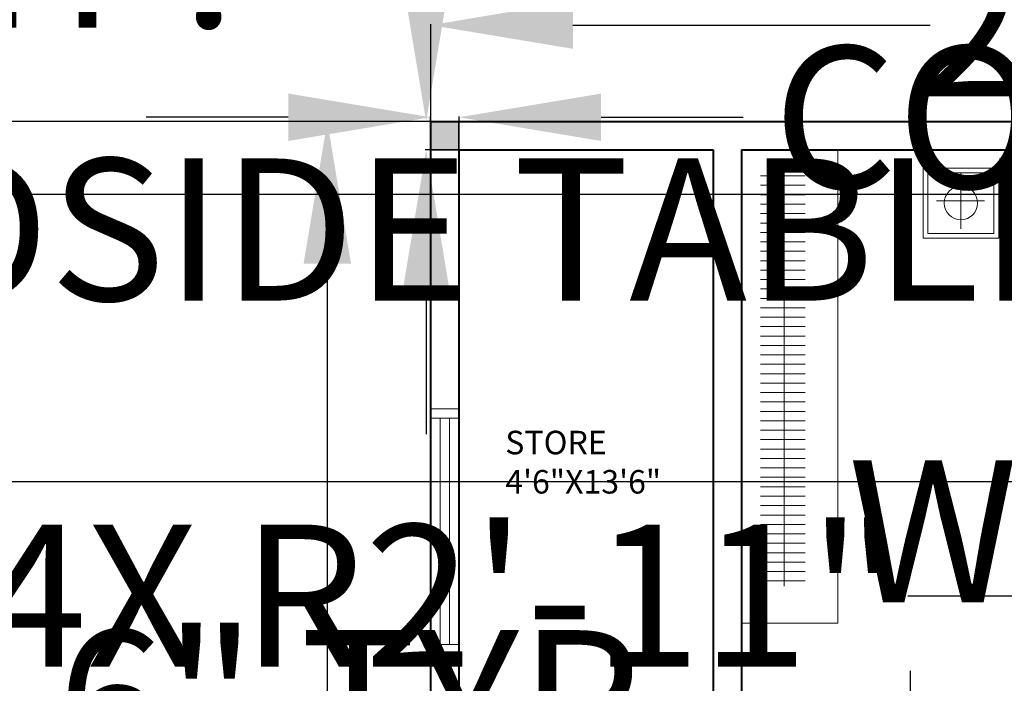
# Model space of a CAD drawing. Units: inches. Extents: x 7323 to 9737, y 2037 to 3322.
# Tile 12 of 19: x 8921 to 9130, y 2568 to 2709. Entities that reach past the tile are written whole.
import ezdxf

# ---------------------------------------------------------------- set-up
doc = ezdxf.new("R2010")
doc.units = ezdxf.units.IN
doc.header["$MEASUREMENT"] = 0
for name, color, linetype, lineweight in [('A-ANNO-DIMS', 2, 'Continuous', 18), ('A-AREA-IDEN', 7, 'Continuous', 18), ('A-COLS', 1, 'Continuous', 35), ('A-FLOR-CASE', 9, 'Continuous', 20), ('A-FLOR-CASE-PATT', 8, 'Continuous', 13), ('A-FURN', 8, 'Continuous', 18), ('A-GLAZ', 4, 'Continuous', 18), ('A-WALL', 7, 'Continuous', 40)]:
    doc.layers.add(name, color=color, linetype=linetype, lineweight=lineweight)
doc.layers.add('A-COLS-PATT', color=18, linetype='Continuous', lineweight=13, true_color=0x000000)
doc.styles.get("Standard").update_dxf_attribs({"font": 'arial.ttf'})
doc.dimstyles.get("Standard").update_dxf_attribs({"dimtxt": 30.18, "dimasz": 30.18, "dimexe": 0.18, "dimexo": 0.0625, "dimgap": 0.09, "dimtad": 0, "dimtih": 1, "dimtoh": 1, "dimdec": 0, "dimzin": 0, "dimdsep": 46, "dimlunit": 3, "dimtxsty": 'Standard', "dimcen": 0.09, "dimadec": 0, "dimazin": 0, "dimtfac": 1, "dimtdec": 0, "dimtofl": 0, "dimtmove": 0, "dimatfit": 3, "dimfxl": 1, "dimtolj": 1, "dimtzin": 0, "dimarcsym": 0})

# ---------------------------------------------------------------- blocks, each defined once
blk = doc.blocks.new('*D10')
at = {"layer": 'A-ANNO-DIMS', "color": 0, "lineweight": -2, "transparency": 16777216}
for p, q in [((9007.95, 2687.36), (9007.95, 2707.94)), ((9038.13, 2707.76), (9113.99, 2707.76)), ((9241.77, 2707.76), (9165.9, 2707.76)), ((9271.95, 2687.36), (9271.95, 2707.94))]:
    blk.add_line(p, q, dxfattribs=at)
at = {"layer": 'A-ANNO-DIMS', "color": 0, "transparency": 16777216}
for points in [[(9038.13, 2712.79), (9038.13, 2702.73), (9007.95, 2707.76)], [(9241.77, 2712.79), (9241.77, 2702.73), (9271.95, 2707.76)]]:
    blk.add_solid(points, dxfattribs=at)
at = {"layer": 'Defpoints', "color": 0, "transparency": 16777216}
for p in [(9271.95, 2707.76), (9007.95, 2687.3), (9271.95, 2687.3)]:
    blk.add_point(p, dxfattribs=at)
at = {"layer": 'A-ANNO-DIMS', "color": 0, "transparency": 16777216, "insert": (9139.95, 2707.76), "char_height": 30.18, "attachment_point": 5}
blk.add_mtext("\\A1;22'", dxfattribs=at)
blk = doc.blocks.new('*D11')
at = {"layer": 'A-ANNO-DIMS', "color": 0, "lineweight": -2, "transparency": 16777216}
for p, q in [((9007.88, 2687.3), (8985.8, 2687.3)), ((8985.98, 2657.12), (8985.98, 2458.79)), ((8985.98, 2229.48), (8985.98, 2427.8)), ((9007.88, 2199.3), (8985.8, 2199.3))]:
    blk.add_line(p, q, dxfattribs=at)
at = {"layer": 'A-ANNO-DIMS', "color": 0, "transparency": 16777216}
for points in [[(8980.95, 2657.12), (8991.01, 2657.12), (8985.98, 2687.3)], [(8980.95, 2229.48), (8991.01, 2229.48), (8985.98, 2199.3)]]:
    blk.add_solid(points, dxfattribs=at)
at = {"layer": 'Defpoints', "color": 0, "transparency": 16777216}
for p in [(9007.95, 2687.3), (8985.98, 2199.3), (9007.95, 2199.3)]:
    blk.add_point(p, dxfattribs=at)
at = {"layer": 'A-ANNO-DIMS', "color": 0, "transparency": 16777216, "insert": (8985.98, 2443.3), "char_height": 30.18, "attachment_point": 5}
blk.add_mtext('\\A1;40\'-8"', dxfattribs=at)
blk = doc.blocks.new('WIN-48')
for p, q in [((0, 0), (0, 6)), ((2, 0), (2, 6)), ((50, 0), (50, 6)), ((52, 0), (52, 6)), ((2, 4), (50, 4)), ((2, 2), (50, 2))]:
    blk.add_line(p, q)
blk = doc.blocks.new('BEDSIDE-TABLE-LARGE')
for p, q in [((8.01, 13.84), (8.01, 1.98)), ((2.84, 7.91), (13.05, 7.91))]:
    blk.add_line(p, q)
for points in [[(0, 14.84), (16.03, 14.84), (16.03, 0), (0, 0)], [(1, 13.84), (15.03, 13.84), (15.03, 1), (1, 1)]]:
    blk.add_lwpolyline(points, close=True)
blk.add_circle((8.01, 7.42), 3.54)
blk = doc.blocks.new('COL-PLAN-6IN')
blk.add_lwpolyline([(0, 6), (0, 6), (6.06, 6), (6.06, 6), (6.06, 0), (6.06, 0), (0, 0), (0, 0)], close=True)
blk = doc.blocks.new('*D35')
at = {"layer": 'A-ANNO-DIMS', "color": 0, "lineweight": -2, "transparency": 16777216}
for p, q in [((8977.7, 2688.2), (8947.52, 2688.2)), ((9007.88, 2687.36), (9007.88, 2688.38)), ((9013.95, 2687.36), (9013.95, 2688.38)), ((9044.13, 2688.2), (9074.31, 2688.2))]:
    blk.add_line(p, q, dxfattribs=at)
at = {"layer": 'A-ANNO-DIMS', "color": 0, "transparency": 16777216}
for points in [[(8977.7, 2693.23), (8977.7, 2683.17), (9007.88, 2688.2)], [(9044.13, 2693.23), (9044.13, 2683.17), (9013.95, 2688.2)]]:
    blk.add_solid(points, dxfattribs=at)
at = {"layer": 'Defpoints', "color": 0, "transparency": 16777216}
for p in [(9007.88, 2687.3), (9013.95, 2688.2), (9013.95, 2687.3)]:
    blk.add_point(p, dxfattribs=at)
at = {"layer": 'A-ANNO-DIMS', "color": 0, "transparency": 16777216, "insert": (9263.41, 2688.2), "char_height": 30.18, "attachment_point": 5}
blk.add_mtext('\\A1;COLUMN 0\'-6" TYP.', dxfattribs=at)
blk = doc.blocks.new('*D36')
at = {"layer": 'A-ANNO-DIMS', "color": 0, "lineweight": -2, "transparency": 16777216}
for p, q in [((9006.97, 2717.48), (9006.97, 2747.66)), ((9006.97, 2747.66), (9037.15, 2747.66)), ((9007.82, 2687.3), (9006.79, 2687.3)), ((9007.82, 2681.3), (9006.79, 2681.3)), ((9006.97, 2651.12), (9006.97, 2620.94))]:
    blk.add_line(p, q, dxfattribs=at)
at = {"layer": 'A-ANNO-DIMS', "color": 0, "transparency": 16777216}
for points in [[(9001.94, 2717.48), (9012, 2717.48), (9006.97, 2687.3)], [(9001.94, 2651.12), (9012, 2651.12), (9006.97, 2681.3)]]:
    blk.add_solid(points, dxfattribs=at)
at = {"layer": 'Defpoints', "color": 0, "transparency": 16777216}
for p in [(9006.97, 2687.3), (9007.88, 2687.3), (9007.88, 2681.3)]:
    blk.add_point(p, dxfattribs=at)
at = {"layer": 'A-ANNO-DIMS', "color": 0, "transparency": 16777216, "insert": (9129.22, 2747.66), "char_height": 30.18, "attachment_point": 5}
blk.add_mtext('\\A1;0\'-6" TYP.', dxfattribs=at)
blk = doc.blocks.new('*D37')
at = {"layer": 'A-ANNO-DIMS', "color": 0, "lineweight": -2, "transparency": 16777216}
for p, q in [((9279.75, 2656.48), (9279.75, 2686.66)), ((9272.01, 2626.3), (9279.93, 2626.3)), ((9272.01, 2574.3), (9279.93, 2574.3)), ((9279.75, 2544.12), (9279.75, 2513.94))]:
    blk.add_line(p, q, dxfattribs=at)
at = {"layer": 'A-ANNO-DIMS', "color": 0, "transparency": 16777216}
for points in [[(9274.72, 2656.48), (9284.78, 2656.48), (9279.75, 2626.3)], [(9274.72, 2544.12), (9284.78, 2544.12), (9279.75, 2574.3)]]:
    blk.add_solid(points, dxfattribs=at)
at = {"layer": 'Defpoints', "color": 0, "transparency": 16777216}
for p in [(9271.95, 2626.3), (9271.95, 2574.3), (9279.75, 2574.3)]:
    blk.add_point(p, dxfattribs=at)
at = {"layer": 'A-ANNO-DIMS', "color": 0, "transparency": 16777216, "insert": (9279.75, 2600.3), "char_height": 30.18, "attachment_point": 5}
blk.add_mtext('\\A1;WINDOW 4\'-4" TYP.', dxfattribs=at)
blk = doc.blocks.new('*D39')
at = {"layer": 'A-ANNO-DIMS', "color": 0, "lineweight": -2, "transparency": 16777216}
for p, q in [((8647.94, 2549.03), (8617.76, 2549.03)), ((8678.12, 2543.2), (8678.12, 2549.21)), ((8717.39, 2543.2), (8717.39, 2549.21)), ((8747.57, 2549.03), (8777.75, 2549.03))]:
    blk.add_line(p, q, dxfattribs=at)
at = {"layer": 'A-ANNO-DIMS', "color": 0, "transparency": 16777216}
for points in [[(8647.94, 2554.06), (8647.94, 2544), (8678.12, 2549.03)], [(8747.57, 2554.06), (8747.57, 2544), (8717.39, 2549.03)]]:
    blk.add_solid(points, dxfattribs=at)
at = {"layer": 'Defpoints', "color": 0, "transparency": 16777216}
for p in [(8717.39, 2549.03), (8678.12, 2543.14), (8717.39, 2543.14)]:
    blk.add_point(p, dxfattribs=at)
at = {"layer": 'A-ANNO-DIMS', "color": 0, "transparency": 16777216, "insert": (9057.19, 2549.03), "char_height": 30.18, "attachment_point": 5}
blk.add_mtext('\\A1;SINGLE DOOR 3\'-3 1/2" TYP.', dxfattribs=at)
blk = doc.blocks.new('*D45')
at = {"layer": 'A-ANNO-DIMS', "color": 0, "lineweight": -2, "transparency": 16777216}
for p, q in [((8725.79, 2664.36), (8695.61, 2664.36)), ((8755.97, 2662.02), (8755.97, 2664.54)), ((8772, 2662.02), (8772, 2664.54)), ((8802.18, 2664.36), (8832.36, 2664.36))]:
    blk.add_line(p, q, dxfattribs=at)
at = {"layer": 'A-ANNO-DIMS', "color": 0, "transparency": 16777216}
for points in [[(8725.79, 2669.39), (8725.79, 2659.33), (8755.97, 2664.36)], [(8802.18, 2669.39), (8802.18, 2659.33), (8772, 2664.36)]]:
    blk.add_solid(points, dxfattribs=at)
at = {"layer": 'Defpoints', "color": 0, "transparency": 16777216}
for p in [(8772, 2664.36), (8755.97, 2661.96), (8772, 2661.96)]:
    blk.add_point(p, dxfattribs=at)
at = {"layer": 'A-ANNO-DIMS', "color": 0, "transparency": 16777216, "insert": (9094.8, 2664.36), "char_height": 30.18, "attachment_point": 5}
blk.add_mtext('\\A1;BEDSIDE TABLE 1\'-4" TYP.', dxfattribs=at)
blk = doc.blocks.new('*D46')
at = {"layer": 'A-ANNO-DIMS', "color": 0, "lineweight": -2, "transparency": 16777216}
for p, q in [((8753.57, 2692.14), (8753.57, 2722.32)), ((8753.57, 2722.32), (8783.75, 2722.32)), ((8755.91, 2661.96), (8753.39, 2661.96)), ((8755.91, 2647.12), (8753.39, 2647.12)), ((8753.57, 2616.94), (8753.57, 2586.76))]:
    blk.add_line(p, q, dxfattribs=at)
at = {"layer": 'A-ANNO-DIMS', "color": 0, "transparency": 16777216}
for points in [[(8748.54, 2692.14), (8758.6, 2692.14), (8753.57, 2661.96)], [(8748.54, 2616.94), (8758.6, 2616.94), (8753.57, 2647.12)]]:
    blk.add_solid(points, dxfattribs=at)
at = {"layer": 'Defpoints', "color": 0, "transparency": 16777216}
for p in [(8753.57, 2661.96), (8755.97, 2661.96), (8755.97, 2647.12)]:
    blk.add_point(p, dxfattribs=at)
at = {"layer": 'A-ANNO-DIMS', "color": 0, "transparency": 16777216, "insert": (8874.4, 2722.32), "char_height": 30.18, "attachment_point": 5}
blk.add_mtext('\\A1;1\'-3" TYP.', dxfattribs=at)
blk = doc.blocks.new('*D52')
at = {"layer": 'A-ANNO-DIMS', "color": 0, "lineweight": -2, "transparency": 16777216}
for p, q in [((9220.65, 2583.03), (9220.65, 2613.21)), ((9209.01, 2552.85), (9220.83, 2552.85)), ((9209.01, 2513.3), (9220.83, 2513.3)), ((9220.65, 2483.12), (9220.65, 2452.94))]:
    blk.add_line(p, q, dxfattribs=at)
at = {"layer": 'A-ANNO-DIMS', "color": 0, "transparency": 16777216}
for points in [[(9215.62, 2583.03), (9225.68, 2583.03), (9220.65, 2552.85)], [(9215.62, 2483.12), (9225.68, 2483.12), (9220.65, 2513.3)]]:
    blk.add_solid(points, dxfattribs=at)
at = {"layer": 'Defpoints', "color": 0, "transparency": 16777216}
for p in [(9208.95, 2552.85), (9220.65, 2552.85), (9208.95, 2513.3)]:
    blk.add_point(p, dxfattribs=at)
at = {"layer": 'A-ANNO-DIMS', "color": 0, "transparency": 16777216, "insert": (9220.65, 2533.07), "char_height": 30.18, "attachment_point": 5}
blk.add_mtext('\\A1;3\'-3 1/2" TYP.', dxfattribs=at)
blk = doc.blocks.new('*D53')
at = {"layer": 'A-ANNO-DIMS', "color": 0, "lineweight": -2, "transparency": 16777216}
for p, q in [((8857.03, 2503.93), (8857.03, 2511.24)), ((8905.03, 2503.93), (8905.03, 2511.24)), ((8826.85, 2511.06), (8796.67, 2511.06)), ((8935.21, 2511.06), (8965.39, 2511.06))]:
    blk.add_line(p, q, dxfattribs=at)
at = {"layer": 'A-ANNO-DIMS', "color": 0, "transparency": 16777216}
for points in [[(8826.85, 2516.09), (8826.85, 2506.03), (8857.03, 2511.06)], [(8935.21, 2516.09), (8935.21, 2506.03), (8905.03, 2511.06)]]:
    blk.add_solid(points, dxfattribs=at)
at = {"layer": 'Defpoints', "color": 0, "transparency": 16777216}
for p in [(8905.03, 2511.06), (8857.03, 2503.86), (8905.03, 2503.86)]:
    blk.add_point(p, dxfattribs=at)
at = {"layer": 'A-ANNO-DIMS', "color": 0, "transparency": 16777216, "insert": (9261.3, 2511.06), "char_height": 30.18, "attachment_point": 5}
blk.add_mtext('\\A1;INTERIOR WINDOW 4\'-0" TYP.', dxfattribs=at)
blk = doc.blocks.new('*D54')
at = {"layer": 'A-ANNO-DIMS', "color": 0, "lineweight": -2, "transparency": 16777216}
for p, q in [((8849.83, 2534.04), (8849.83, 2564.22)), ((8849.83, 2564.22), (8880.01, 2564.22)), ((8856.96, 2503.86), (8849.65, 2503.86)), ((8856.96, 2497.86), (8849.65, 2497.86)), ((8849.83, 2467.68), (8849.83, 2437.5))]:
    blk.add_line(p, q, dxfattribs=at)
at = {"layer": 'A-ANNO-DIMS', "color": 0, "transparency": 16777216}
for points in [[(8844.8, 2534.04), (8854.86, 2534.04), (8849.83, 2503.86)], [(8844.8, 2467.68), (8854.86, 2467.68), (8849.83, 2497.86)]]:
    blk.add_solid(points, dxfattribs=at)
at = {"layer": 'Defpoints', "color": 0, "transparency": 16777216}
for p in [(8849.83, 2503.86), (8857.03, 2503.86), (8857.03, 2497.86)]:
    blk.add_point(p, dxfattribs=at)
at = {"layer": 'A-ANNO-DIMS', "color": 0, "transparency": 16777216, "insert": (8972.08, 2564.22), "char_height": 30.18, "attachment_point": 5}
blk.add_mtext('\\A1;0\'-6" TYP.', dxfattribs=at)
blk = doc.blocks.new('*D59')
at = {"layer": 'A-ANNO-DIMS', "color": 0, "lineweight": -2, "transparency": 16777216}
for p, q in [((9064.67, 2473.96), (9064.67, 2467.95)), ((9103.95, 2473.96), (9103.95, 2467.95)), ((9034.49, 2468.13), (9004.31, 2468.13)), ((9134.13, 2468.13), (9164.31, 2468.13))]:
    blk.add_line(p, q, dxfattribs=at)
at = {"layer": 'A-ANNO-DIMS', "color": 0, "transparency": 16777216}
for points in [[(9034.49, 2473.16), (9034.49, 2463.1), (9064.67, 2468.13)], [(9134.13, 2473.16), (9134.13, 2463.1), (9103.95, 2468.13)]]:
    blk.add_solid(points, dxfattribs=at)
at = {"layer": 'Defpoints', "color": 0, "transparency": 16777216}
for p in [(9064.67, 2474.02), (9103.95, 2474.02), (9103.95, 2468.13)]:
    blk.add_point(p, dxfattribs=at)
at = {"layer": 'A-ANNO-DIMS', "color": 0, "transparency": 16777216, "insert": (9458.35, 2468.13), "char_height": 30.18, "attachment_point": 5}
blk.add_mtext('\\A1;KITCHEN DOOR 3\'-3 1/2" TYP.', dxfattribs=at)
blk = doc.blocks.new('*D60')
at = {"layer": 'A-ANNO-DIMS', "color": 0, "lineweight": -2, "transparency": 16777216}
for p, q in [((9109.84, 2540.48), (9109.84, 2570.66)), ((9104.01, 2510.3), (9110.02, 2510.3)), ((9104.01, 2474.02), (9110.02, 2474.02)), ((9109.84, 2443.84), (9109.84, 2413.66))]:
    blk.add_line(p, q, dxfattribs=at)
at = {"layer": 'A-ANNO-DIMS', "color": 0, "transparency": 16777216}
for points in [[(9104.81, 2540.48), (9114.87, 2540.48), (9109.84, 2510.3)], [(9104.81, 2443.84), (9114.87, 2443.84), (9109.84, 2474.02)]]:
    blk.add_solid(points, dxfattribs=at)
at = {"layer": 'Defpoints', "color": 0, "transparency": 16777216}
for p in [(9103.95, 2510.3), (9109.84, 2510.3), (9103.95, 2474.02)]:
    blk.add_point(p, dxfattribs=at)
at = {"layer": 'A-ANNO-DIMS', "color": 0, "transparency": 16777216, "insert": (9109.84, 2492.16), "char_height": 30.18, "attachment_point": 5}
blk.add_mtext('\\A1;3\'-0 1/2" TYP.', dxfattribs=at)
blk = doc.blocks.new('*D65')
at = {"layer": 'A-ANNO-DIMS', "color": 0, "lineweight": -2, "transparency": 16777216}
for p, q in [((9024.02, 2513.3), (9024.02, 2543.48)), ((9024.02, 2543.48), (9054.2, 2543.48)), ((9036.56, 2513.3), (9023.84, 2513.3)), ((9024.02, 2459.48), (9024.02, 2483.12)), ((9036.56, 2429.3), (9023.84, 2429.3))]:
    blk.add_line(p, q, dxfattribs=at)
at = {"layer": 'A-ANNO-DIMS', "color": 0, "transparency": 16777216}
for points in [[(9018.99, 2483.12), (9029.05, 2483.12), (9024.02, 2513.3)], [(9018.99, 2459.48), (9029.05, 2459.48), (9024.02, 2429.3)]]:
    blk.add_solid(points, dxfattribs=at)
at = {"layer": 'Defpoints', "color": 0, "transparency": 16777216}
for p in [(9024.02, 2513.3), (9036.62, 2513.3), (9036.62, 2429.3)]:
    blk.add_point(p, dxfattribs=at)
at = {"layer": 'A-ANNO-DIMS', "color": 0, "transparency": 16777216, "insert": (9256.18, 2543.48), "char_height": 30.18, "attachment_point": 5}
blk.add_mtext('\\A1;COUNTER 7\'-0" TYP.', dxfattribs=at)
blk = doc.blocks.new('*D66')
at = {"layer": 'A-ANNO-DIMS', "color": 0, "lineweight": -2, "transparency": 16777216}
for p, q in [((9006.44, 2525.9), (8976.26, 2525.9)), ((9036.62, 2513.36), (9036.62, 2526.08)), ((9075.95, 2513.36), (9075.95, 2526.08)), ((9106.13, 2525.9), (9136.31, 2525.9))]:
    blk.add_line(p, q, dxfattribs=at)
at = {"layer": 'A-ANNO-DIMS', "color": 0, "transparency": 16777216}
for points in [[(9006.44, 2530.93), (9006.44, 2520.87), (9036.62, 2525.9)], [(9106.13, 2530.93), (9106.13, 2520.87), (9075.95, 2525.9)]]:
    blk.add_solid(points, dxfattribs=at)
at = {"layer": 'Defpoints', "color": 0, "transparency": 16777216}
for p in [(9075.95, 2525.9), (9036.62, 2513.3), (9075.95, 2513.3)]:
    blk.add_point(p, dxfattribs=at)
at = {"layer": 'A-ANNO-DIMS', "color": 0, "transparency": 16777216, "insert": (9263.53, 2525.9), "char_height": 30.18, "attachment_point": 5}
blk.add_mtext('\\A1;3\'-3 1/2" TYP.', dxfattribs=at)
blk = doc.blocks.new('*D69')
at = {"layer": 'A-ANNO-DIMS', "color": 0, "lineweight": -2, "transparency": 16777216}
for p, q in [((8836.58, 2472.89), (8836.58, 2503.07)), ((8836.58, 2503.07), (8866.76, 2503.07)), ((8839.88, 2442.71), (8836.4, 2442.71)), ((8839.88, 2420.33), (8836.4, 2420.33)), ((8836.58, 2390.15), (8836.58, 2359.97))]:
    blk.add_line(p, q, dxfattribs=at)
at = {"layer": 'A-ANNO-DIMS', "color": 0, "transparency": 16777216}
for points in [[(8831.55, 2472.89), (8841.61, 2472.89), (8836.58, 2442.71)], [(8831.55, 2390.15), (8841.61, 2390.15), (8836.58, 2420.33)]]:
    blk.add_solid(points, dxfattribs=at)
at = {"layer": 'Defpoints', "color": 0, "transparency": 16777216}
for p in [(8836.58, 2442.71), (8839.94, 2442.71), (8839.94, 2420.33)]:
    blk.add_point(p, dxfattribs=at)
at = {"layer": 'A-ANNO-DIMS', "color": 0, "transparency": 16777216, "insert": (9169.54, 2503.07), "char_height": 30.18, "attachment_point": 5}
blk.add_mtext('\\A1;COFFEE TABLE 1\'-10 1/2" TYP.', dxfattribs=at)
blk = doc.blocks.new('*D100')
at = {"layer": 'A-ANNO-DIMS', "color": 0, "lineweight": -2, "transparency": 16777216}
for p, q in [((9007.88, 2687.3), (8587.16, 2687.3)), ((8587.34, 2657.12), (8587.34, 2615.8)), ((8587.34, 2543.49), (8587.34, 2584.8)), ((9008.12, 2513.31), (8587.16, 2513.31))]:
    blk.add_line(p, q, dxfattribs=at)
at = {"layer": 'A-ANNO-DIMS', "color": 0, "transparency": 16777216}
for points in [[(8582.31, 2657.12), (8592.37, 2657.12), (8587.34, 2687.3)], [(8582.31, 2543.49), (8592.37, 2543.49), (8587.34, 2513.31)]]:
    blk.add_solid(points, dxfattribs=at)
at = {"layer": 'Defpoints', "color": 0, "transparency": 16777216}
for p in [(9007.95, 2687.3), (8587.34, 2513.31), (9008.18, 2513.31)]:
    blk.add_point(p, dxfattribs=at)
at = {"layer": 'A-ANNO-DIMS', "color": 0, "transparency": 16777216, "insert": (8587.34, 2600.3), "char_height": 30.18, "attachment_point": 5}
blk.add_mtext('\\A1;14\'-6"', dxfattribs=at)
blk = doc.blocks.new('*D114')
at = {"layer": 'A-ANNO-DIMS', "color": 0, "lineweight": -2, "transparency": 16777216}
for p, q in [((8915.46, 2671.86), (9307.45, 2671.86)), ((9307.27, 2641.68), (9307.27, 2641.04)), ((8915.46, 2610.86), (9307.45, 2610.86)), ((9307.27, 2610.86), (9307.27, 2580.68)), ((9307.27, 2580.68), (9277.09, 2580.68))]:
    blk.add_line(p, q, dxfattribs=at)
at = {"layer": 'A-ANNO-DIMS', "color": 0, "transparency": 16777216}
for points in [[(9302.24, 2641.68), (9312.3, 2641.68), (9307.27, 2671.86)], [(9302.24, 2641.04), (9312.3, 2641.04), (9307.27, 2610.86)]]:
    blk.add_solid(points, dxfattribs=at)
at = {"layer": 'Defpoints', "color": 0, "transparency": 16777216}
for p in [(8915.39, 2671.86), (8915.39, 2610.86), (9307.27, 2610.86)]:
    blk.add_point(p, dxfattribs=at)
at = {"layer": 'A-ANNO-DIMS', "color": 0, "transparency": 16777216, "insert": (9236.89, 2580.68), "char_height": 30.18, "attachment_point": 5}
blk.add_mtext('\\A1;5\'-1"', dxfattribs=at)
blk = doc.blocks.new('*D126')
at = {"layer": 'A-ANNO-DIMS', "color": 0, "lineweight": -2, "transparency": 16777216}
for p, q in [((9109.28, 2586.63), (9139.46, 2586.63)), ((9139.46, 2586.63), (9160.18, 2564.69)), ((9204.86, 2517.3), (9205.04, 2517.3)), ((9204.95, 2517.21), (9204.95, 2517.39))]:
    blk.add_line(p, q, dxfattribs=at)
at = {"layer": 'A-ANNO-DIMS', "color": 0, "transparency": 16777216}
blk.add_solid([(9163.84, 2568.15), (9156.52, 2561.24), (9180.9, 2542.75)], dxfattribs=at)
at = {"layer": 'Defpoints', "color": 0, "transparency": 16777216}
for p in [(9180.9, 2542.75), (9204.95, 2517.3)]:
    blk.add_point(p, dxfattribs=at)
at = {"layer": 'A-ANNO-DIMS', "color": 0, "transparency": 16777216, "insert": (9009.88, 2586.63), "char_height": 30.18, "attachment_point": 5}
blk.add_mtext('\\A1;4X R2\'-11"', dxfattribs=at)

msp = doc.modelspace()

# ---------------------------------------------------------------- hatches: boundary and pattern name
at = {"layer": 'A-COLS-PATT'}
h = msp.add_hatch(color=256, dxfattribs=at)
h.dxf.hatch_style = 1
h.paths.add_polyline_path([(8915.39, 2189.86), (8908.77, 2189.86), (8908.77, 2183.86), (8915.39, 2183.86)])
h.paths.add_polyline_path([(8657.61, 2189.86), (8651.55, 2189.86), (8651.55, 2183.86), (8657.61, 2183.86)])
h.paths.add_polyline_path([(8814.13, 2189.86), (8807.39, 2189.86), (8807.39, 2183.86), (8814.13, 2183.86)])
h.paths.add_polyline_path([(8813.39, 2317.86), (8807.36, 2317.86), (8807.36, 2311.86), (8813.39, 2311.86)])
h.paths.add_polyline_path([(8915.34, 2313.13), (8909.39, 2313.13), (8909.39, 2307.13), (8915.34, 2307.13)])
h.paths.add_polyline_path([(8657.62, 2317.86), (8657.39, 2317.86), (8657.39, 2318.08), (8651.55, 2318.08), (8651.55, 2312.08), (8657.62, 2312.08)])
h.paths.add_polyline_path([(8915.39, 2671.84), (8909.37, 2671.84), (8909.37, 2665.86), (8909.39, 2665.86), (8915.39, 2665.84)])
h.paths.add_polyline_path([(8657.59, 2671.81), (8651.52, 2671.81), (8651.52, 2665.81), (8657.39, 2665.81), (8657.39, 2665.86)])
h.paths.add_polyline_path([(8915.28, 2503.94), (8909.39, 2503.94), (8909.39, 2503.86), (8909.22, 2497.94), (8915.28, 2497.94)])
h.paths.add_polyline_path([(8657.53, 2503.86), (8657.39, 2503.86), (8651.46, 2503.96), (8651.46, 2497.96), (8657.53, 2497.96)])
h.paths.add_polyline_path([(9014.24, 2519.3), (9013.95, 2519.3), (9008.18, 2519.31), (9008.18, 2513.31), (9014.24, 2513.31)])
h.paths.add_polyline_path([(9013.95, 2687.3), (9007.95, 2687.3), (9007.95, 2681.3), (9013.95, 2681.3)])
h.paths.add_polyline_path([(9271.95, 2687.3), (9266.01, 2687.3), (9266.01, 2681.35), (9271.95, 2681.35)])
h.paths.add_polyline_path([(9271.95, 2205.3), (9265.32, 2205.3), (9265.32, 2199.3), (9271.95, 2199.3)])
h.paths.add_polyline_path([(9170.68, 2205.3), (9163.95, 2205.3), (9163.95, 2199.3), (9170.68, 2199.3)])
h.paths.add_polyline_path([(9013.95, 2205.3), (9007.95, 2205.3), (9007.95, 2199.3), (9013.95, 2199.3)])
h.paths.add_polyline_path([(9271.95, 2519.51), (9265.95, 2519.51), (9265.95, 2519.3), (9265.93, 2513.51), (9271.95, 2513.51)])
h.paths.add_polyline_path([(9271.95, 2328.64), (9265.95, 2328.64), (9265.95, 2322.64), (9271.95, 2322.64)])
h.paths.add_polyline_path([(9014.35, 2333.3), (9013.95, 2333.3), (9013.95, 2333.58), (9008.29, 2333.58), (9008.29, 2327.58), (9014.35, 2327.58)])
at = {"layer": 'A-FLOR-CASE-PATT'}
h = msp.add_hatch(dxfattribs=at)
h.set_pattern_fill('ANSI31', color=256, scale=15.998486, angle=-45, style=0)
h.paths.add_polyline_path([(9077.96, 2589.72), (9087.46, 2589.72), (9087.46, 2675.78), (9077.96, 2675.78)])

# ---------------------------------------------------------------- linework, layer by layer
at = {"layer": 'A-FLOR-CASE'}
msp.add_line((9082.98, 2677.66), (9082.98, 2588.63), dxfattribs=at)
msp.add_lwpolyline([(9073.95, 2681.3), (9094.37, 2681.3), (9094.37, 2580.82), (9073.95, 2580.82)], close=True, dxfattribs=at)
at = {"layer": 'A-WALL'}
for p, q in [((9007.95, 2199.3), (9007.95, 2687.3)), ((9007.95, 2687.3), (9271.95, 2687.3)), ((9013.95, 2519.3), (9013.95, 2681.3)), ((9013.95, 2681.3), (9067.95, 2681.3)), ((9067.95, 2681.3), (9067.95, 2558.25)), ((9073.95, 2681.3), (9265.95, 2681.3)), ((9073.95, 2681.3), (9073.95, 2558.3))]:
    msp.add_line(p, q, dxfattribs=at)

# ---------------------------------------------------------------- block references
at = {"layer": 'A-COLS'}
msp.add_blockref('COL-PLAN-6IN', (9007.88, 2681.3), dxfattribs=at)
at = {"layer": 'A-FURN'}
msp.add_blockref('BEDSIDE-TABLE-LARGE', (9112.52, 2662.55), dxfattribs=at)
at = {"layer": 'A-GLAZ', "rotation": 270.0000000000041}
msp.add_blockref('WIN-48', (9007.95, 2626.29), dxfattribs=at)

# ---------------------------------------------------------------- texts
at = {"layer": 'A-AREA-IDEN', "insert": (9023.77, 2621.64), "char_height": 5, "attachment_point": 1}
msp.add_mtext_dynamic_manual_height_columns('STORE\\P4\'6"X13\'6"', width=44.1759, gutter_width=1, heights=[0], dxfattribs=at)

# ---------------------------------------------------------------- dimensions: what is measured, and where the dimension line sits
at = {"layer": 'A-ANNO-DIMS'}
for base, p1, p2, angle, text, picture, middle in [((9006.97, 2687.3), (9007.88, 2681.3), (9007.88, 2687.3), 90, '<> TYP.', '*D36', (9129.22, 2747.66)), ((8753.57, 2661.96), (8755.97, 2647.12), (8755.97, 2661.96), 90, '<> TYP.', '*D46', (8874.4, 2722.32)), ((9279.75, 2574.3), (9271.95, 2626.3), (9271.95, 2574.3), 270, 'WINDOW <> TYP.', '*D37', (9279.75, 2600.3)), ((8836.58, 2442.71), (8839.94, 2420.33), (8839.94, 2442.71), 90, 'COFFEE TABLE <> TYP.', '*D69', (9169.54, 2503.07)), ((9024.02, 2513.3), (9036.62, 2429.3), (9036.62, 2513.3), 90, 'COUNTER <> TYP.', '*D65', (9256.18, 2543.48)), ((9220.6454, 2552.8475), (9208.9454, 2513.2952), (9208.9454, 2552.8475), 90, '<> TYP.', '*D52', (9220.6454, 2533.0713)), ((8849.83, 2503.86), (8857.03, 2497.86), (8857.03, 2503.86), 90, '<> TYP.', '*D54', (8972.08, 2564.22)), ((9109.84, 2510.3), (9103.95, 2474.02), (9103.95, 2510.3), 90, '<> TYP.', '*D60', (9109.84, 2492.16))]:
    dim = msp.add_linear_dim(base=base, p1=p1, p2=p2, angle=angle, text=text, dimstyle='Standard', override={"dimdec": 1, "dimlfac": 1, "dimrnd": 0, "dimzin": 1, "dimdsep": 46, "dimlunit": 4, "dimfrac": 2}, dxfattribs=at)
    dim.commit()
    dim.dimension.update_dxf_attribs({"geometry": picture, "text_midpoint": middle})
for base, p1, p2, text, picture, middle in [((8772, 2664.36), (8755.97, 2661.96), (8772, 2661.96), 'BEDSIDE TABLE <> TYP.', '*D45', (9094.8, 2664.36)), ((9013.95, 2688.2), (9007.88, 2687.3), (9013.95, 2687.3), 'COLUMN <> TYP.', '*D35', (9263.41, 2688.2)), ((8717.39, 2549.03), (8678.12, 2543.14), (8717.39, 2543.14), 'SINGLE DOOR <> TYP.', '*D39', (9057.19, 2549.03)), ((8905.03, 2511.06), (8857.03, 2503.86), (8905.03, 2503.86), 'INTERIOR WINDOW <> TYP.', '*D53', (9261.3, 2511.06)), ((9075.95, 2525.9), (9036.62, 2513.3), (9075.95, 2513.3), '<> TYP.', '*D66', (9263.53, 2525.9)), ((9103.95, 2468.13), (9064.67, 2474.02), (9103.95, 2474.02), 'KITCHEN DOOR <> TYP.', '*D59', (9458.35, 2468.13))]:
    dim = msp.add_linear_dim(base=base, p1=p1, p2=p2, text=text, dimstyle='Standard', override={"dimdec": 1, "dimlfac": 1, "dimrnd": 0, "dimzin": 1, "dimdsep": 46, "dimlunit": 4, "dimfrac": 2}, dxfattribs=at)
    dim.commit()
    dim.dimension.update_dxf_attribs({"geometry": picture, "text_midpoint": middle})
dim = msp.add_linear_dim(base=(9271.95, 2707.76), p1=(9007.95, 2687.3), p2=(9271.95, 2687.3), dimstyle='Standard', override={"dimclrd": 0, "dimclre": 0, "dimclrt": 0}, dxfattribs=at)
dim.commit()
dim.dimension.update_dxf_attribs({"geometry": '*D10', "text_midpoint": (9139.95, 2707.76)})
for base, p1, p2, override, picture, middle in [((8587.34, 2513.31), (9007.95, 2687.3), (9008.18, 2513.31), {"dimdec": 1, "dimlfac": 1, "dimrnd": 0, "dimzin": 1, "dimdsep": 46, "dimlunit": 4, "dimfrac": 2}, '*D100', (8587.34, 2600.3)), ((8985.98, 2199.3), (9007.95, 2687.3), (9007.95, 2199.3), {"dimclrd": 0, "dimclre": 0, "dimclrt": 0}, '*D11', (8985.98, 2443.3)), ((9307.27, 2610.86), (8915.39, 2671.86), (8915.39, 2610.86), {"dimdec": 1, "dimlfac": 1, "dimrnd": 0, "dimzin": 1, "dimdsep": 46, "dimlunit": 4, "dimfrac": 2}, '*D114', (9236.89, 2580.68))]:
    dim = msp.add_linear_dim(base=base, p1=p1, p2=p2, angle=90, dimstyle='Standard', override=override, dxfattribs=at)
    dim.commit()
    dim.dimension.update_dxf_attribs({"geometry": picture, "text_midpoint": middle})
dim = msp.add_radius_dim(center=(9204.95, 2517.3), mpoint=(9180.9, 2542.75), text='4X <>', dimstyle='Standard', override={"dimdec": 1, "dimlfac": 1, "dimrnd": 0, "dimzin": 1, "dimdsep": 46, "dimlunit": 4, "dimfrac": 2}, dxfattribs=at)
dim.commit()
dim.dimension.update_dxf_attribs({"geometry": '*D126', "text_midpoint": (9009.88, 2586.63)})

doc.saveas('drawing.dxf')
